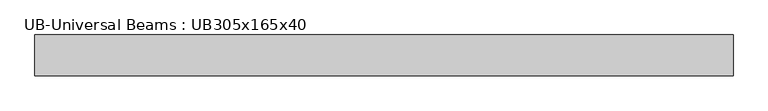
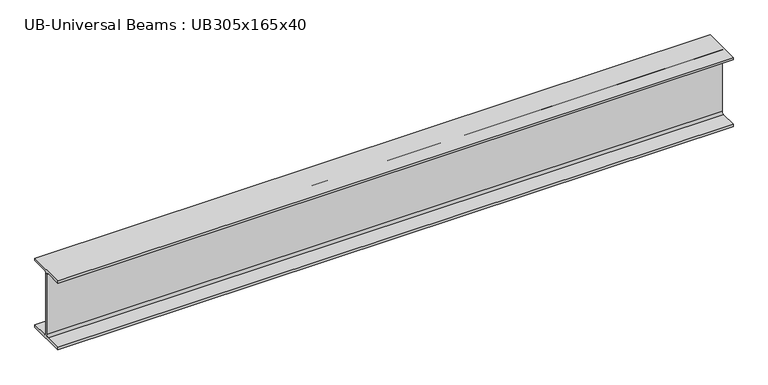
"""IFC4 building model written with IfcOpenShell, lengths in millimetres: beam geometry, UB-Universal Beams : UB305x165x40."""

from ifc_helpers import new_model, si_unit, point, frame, frame_2d, origin, place, context, project, spatial, polyline, circle_curve, trimmed, segment, composite_curve, outline, extrude, source, transform, mapped, element, save


def ub_universal_beams_ub305x165x40_219eb426(model_context):
    return source(origin(), model_context, "Body", "SweptSolid", [
        extrude(outline(composite_curve([segment(polyline([(82.5, -141.5), (82.5, -151.7), (-82.5, -151.7), (-82.5, -141.5), (-11.9, -141.5)]), True, "CONTINUOUS"), segment(trimmed(circle_curve(frame_2d((-11.9, -132.6)), 8.9), [point((-11.9, -141.5))], [point((-3.0, -132.6))], True, "CARTESIAN"), True, "CONTINUOUS"), segment(polyline([(-3.0, -132.6), (-3.0, 132.6)]), True, "CONTINUOUS"), segment(trimmed(circle_curve(frame_2d((-11.9, 132.6)), 8.9), [point((-3.0, 132.6))], [point((-11.9, 141.5))], True, "CARTESIAN"), True, "CONTINUOUS"), segment(polyline([(-11.9, 141.5), (-82.5, 141.5), (-82.5, 151.7), (82.5, 151.7), (82.5, 141.5), (11.9, 141.5)]), True, "CONTINUOUS"), segment(trimmed(circle_curve(frame_2d((11.9, 132.6)), 8.9), [point((11.9, 141.5))], [point((3.0, 132.6))], True, "CARTESIAN"), True, "CONTINUOUS"), segment(polyline([(3.0, 132.6), (3.0, -132.6)]), True, "CONTINUOUS"), segment(trimmed(circle_curve(frame_2d((11.9, -132.6)), 8.9), [point((3.0, -132.6))], [point((11.9, -141.5))], True, "CARTESIAN"), True, "CONTINUOUS"), segment(polyline([(11.9, -141.5), (82.5, -141.5)]), True, "CONTINUOUS")], self_intersect=False)), frame((-1404.8, 0.0, 0.0), z_axis=(1.0, 0.0, 0.0), x_axis=(0.0, 1.0, 0.0)), (0.0, 0.0, 1.0), 2809.6),
    ])


if __name__ == "__main__":
    model = new_model("IFC4")
    model_context = context("Model", 3, world=origin())
    ifc_project = project(units=[si_unit("LENGTHUNIT", "METRE", prefix="MILLI")], contexts=[model_context])
    site = spatial("IfcSite", under=ifc_project)
    building = spatial("IfcBuilding", under=site)
    placement = place(None, origin())
    ub_universal_beams_ub305x165x40_shape = ub_universal_beams_ub305x165x40_219eb426(model_context)
    element("IfcBeam", 1, ObjectType="UB-Universal Beams : UB305x165x40", at=placement, inside=building, context=model_context, shape_type="MappedRepresentation", body=[
        mapped(ub_universal_beams_ub305x165x40_shape, transform((0.0, 0.0, 0.0), x_axis=(1.0, 0.0, 0.0), y_axis=(0.0, 1.0, 0.0), z_axis=(0.0, 0.0, 1.0))),
    ])
    save(model, "model.ifc")

# Revit data of these elements
# Type "UB-Universal Beams : UB305x165x40"
#   Section Name Key = "UB305X165X40"
#   Width = 16.5 cm
#   Web Thickness = 0.6 cm
#   Web Fillet = 0.89 cm
#   Warping Constant = 164000.0 cm⁶
#   Torsional Moment of Inertia = 14.70 cm⁴
#   Section Area = 51.3 cm²
#   Plastic Modulus weak axis = 142.0 cm³
#   Plastic Modulus strong axis = 623.0 cm³
#   Nominal Weight = 40.2999 kgf/m
#   Moment of Inertia weak axis = 764.00 cm⁴
#   Moment of Inertia strong axis = 8503.00 cm⁴
#   Height = 30.34 cm
#   Flange Thickness = 1.02 cm
#   Elastic Modulus weak axis = 92.6 cm³
#   Elastic Modulus strong axis = 560.0 cm³
#   Centroid Vertical = 15.17 cm
#   Centroid Horizontal = 8.25 cm
#   Bolt Spacing = 9.0 cm
#   Length [instance default] = 1.5 m
#   Structural Material [instance default] = Metal - Steel 43-275
#   Type Comments = ""
#   Assembly Code = ""
# Element 1 (IfcBeam, "UB-Universal Beams : UB305x165x40")
#   Materials on its faces: "Metal - Steel 43-275"
# Materials
#   "Metal - Steel 43-275": class "Metal", colour RGB 247 247 247, transparency 0, Cost = 0
